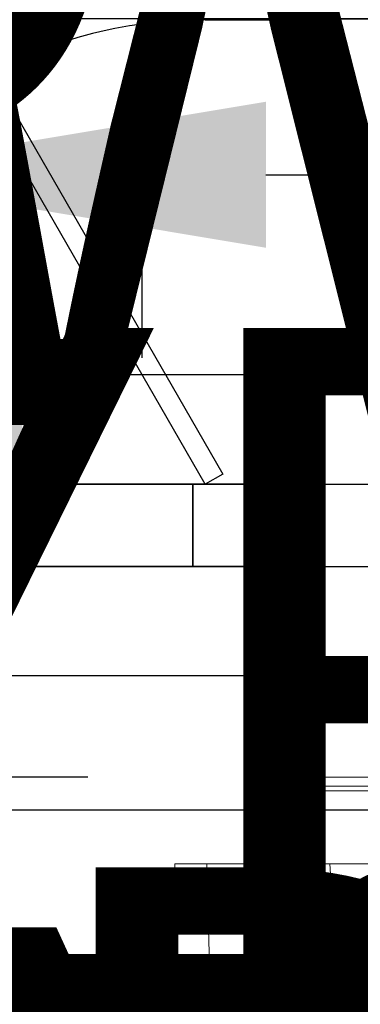
# Model space of a CAD drawing. Units: inches. Extents: x -307 to 2141, y -58 to 895.
# Tile 17 of 28: x 666 to 704, y 481 to 589. Entities that reach past the tile are written whole.
import ezdxf

# ---------------------------------------------------------------- set-up
doc = ezdxf.new("R2010")
doc.units = ezdxf.units.IN
doc.header["$MEASUREMENT"] = 0
for name, color, linetype, lineweight in [('A-ANNO-DIMS', 2, 'Continuous', 18), ('A-DOOR', 3, 'Continuous', 25), ('A-FURN', 8, 'Continuous', 18), ('A-WALL', 7, 'Continuous', 35)]:
    doc.layers.add(name, color=color, linetype=linetype, lineweight=lineweight)
doc.styles.get("Standard").update_dxf_attribs({"font": 'arial.ttf'})
doc.dimstyles.get("Standard").update_dxf_attribs({"dimtxt": 72, "dimasz": 48, "dimexe": 0.18, "dimexo": 0.0625, "dimgap": 0.09, "dimtad": 0, "dimtih": 1, "dimtoh": 1, "dimdec": 0, "dimrnd": 48, "dimzin": 0, "dimdsep": 46, "dimlunit": 3, "dimtxsty": 'Standard', "dimcen": 0.09, "dimadec": 0, "dimazin": 0, "dimtfac": 1, "dimtdec": 0, "dimtofl": 0, "dimtmove": 0, "dimatfit": 3, "dimfxl": 1, "dimtolj": 1, "dimtzin": 0, "dimarcsym": 0})

# ---------------------------------------------------------------- blocks, each defined once
blk = doc.blocks.new('*U3')
for p, q in [((-40, 0), (-40, 6)), ((0, 0), (0, 6))]:
    blk.add_line(p, q)
blk.add_lwpolyline([(0, 0), (-34.641, -20), (-35.516, -18.484), (-0.875, 1.516)], close=True)
blk.add_arc((0, 0), 40, 180, 210)
blk = doc.blocks.new('Dining Set - 36 x 72 in.')
for p, q in [((-22, 27.5), (-22.1562, 26.50042)), ((-22, 27.5), (-6, 27.5)), ((-5.8437, 26.49966), (-6, 27.5)), ((6, 27.5), (5.8438, 26.50042)), ((6, 27.5), (22, 27.5)), ((22.1563, 26.49966), (22, 27.5)), ((-22.2343, 26.00059), (-23.4847, 17.99762)), ((-22.2304, 26), (-5.7608, 26)), ((-5.8416, 26.5), (-22.1534, 26.5)), ((-4.5152, 17.99762), (-5.7655, 25.99926)), ((5.7657, 26.00059), (4.5153, 17.99762)), ((5.7696, 26), (22.2392, 26)), ((22.1584, 26.5), (5.8466, 26.5)), ((23.4848, 17.99762), (22.2345, 25.99926)), ((36, 18), (-36, 18)), ((-36, 18), (-36, -18)), ((36, -18), (36, 18)), ((-44.0006, 8.23428), (-35.9976, 9.48474)), ((44.0006, 8.23428), (35.9976, 9.48474)), ((-45.5, 8), (-44.5004, 8.15617)), ((-45.5, 8), (-45.5, -8)), ((-44.5, -8.15843), (-44.5, 8.15338)), ((-44, 8.23041), (-44, -8.23915)), ((44, 8.23041), (44, -8.23915)), ((44.5, -8.15843), (44.5, 8.15338)), ((45.5, 8), (44.5005, 8.15617)), ((45.5, 8), (45.5, -8)), ((-44.4997, -8.15631), (-45.5, -8)), ((-35.9976, -9.48476), (-43.9993, -8.2345)), ((35.9976, -9.48476), (43.9993, -8.2345)), ((44.4997, -8.15631), (45.5, -8)), ((-36, -18), (36, -18)), ((-22.2343, -26.0006), (-23.4847, -17.99762)), ((-4.5152, -17.99762), (-5.7655, -25.99928)), ((5.7657, -26.0006), (4.5153, -17.99762)), ((23.4848, -17.99762), (22.2345, -25.99928)), ((-22.2304, -26), (-5.7608, -26)), ((-22, -27.5), (-22.1562, -26.50044)), ((-5.8416, -26.5), (-22.1534, -26.5)), ((-5.8437, -26.49967), (-6, -27.5)), ((5.7696, -26), (22.2392, -26)), ((6, -27.5), (5.8438, -26.50044)), ((22.1584, -26.5), (5.8466, -26.5)), ((22.1563, -26.49967), (22, -27.5)), ((-22, -27.5), (-6, -27.5)), ((6, -27.5), (22, -27.5))]:
    blk.add_line(p, q)
for points in [[(-36, 15), (-31.1772, 14.97754), (-26.8079, 14.91406), (-22.8538, 14.81543), (-19.276, 14.6875), (-16.0362, 14.53613), (-13.0957, 14.36718), (-10.4159, 14.18652), (-7.9583, 14), (-5.6904, 13.81315), (-3.6035, 13.63021), (-1.6954, 13.45508), (0.0365, 13.29166), (1.5945, 13.14388), (2.9811, 13.01562), (4.1988, 12.9108), (5.25, 12.83333), (6.1393, 12.78613), (6.8802, 12.76823), (7.4883, 12.77767), (7.9792, 12.8125), (8.3685, 12.87077), (8.6719, 12.95052), (8.9049, 13.0498), (9.0833, 13.16666), (9.2205, 13.29899), (9.3216, 13.44401), (9.3895, 13.59879), (9.4271, 13.76041), (9.4373, 13.92594), (9.4232, 14.09245), (9.3875, 14.257), (9.3333, 14.41666), (9.2638, 14.56917), (9.1836, 14.71484), (9.0975, 14.85465), (9.0104, 14.98958), (8.9272, 15.1206), (8.8529, 15.2487), (8.7922, 15.37483), (8.75, 15.5), (8.7305, 15.62467), (8.7344, 15.74739), (8.7617, 15.86621), (8.8125, 15.97916), (8.8867, 16.08431), (8.9844, 16.17968), (9.1055, 16.26334), (9.25, 16.33333), (9.4189, 16.38802), (9.6172, 16.42708), (9.8506, 16.45052), (10.125, 16.45833), (10.4463, 16.45052), (10.8203, 16.42708), (11.2529, 16.38802), (11.75, 16.33333), (12.3184, 16.26318), (12.9694, 16.17838), (13.7151, 16.07991), (14.5677, 15.96875), (15.5395, 15.84586), (16.6426, 15.71224), (17.8893, 15.56884), (19.2917, 15.41666), (20.859, 15.25667), (22.5879, 15.08984), (24.4721, 14.91715), (26.5052, 14.73958), (28.6809, 14.5581), (30.9929, 14.3737), (33.4347, 14.18733), (36, 14)], [(-36, 10), (-28.9766, 10.14274), (-23.1725, 10.20442), (-18.4241, 10.19775), (-14.5677, 10.13541), (-11.4399, 10.03011), (-8.877, 9.89453), (-6.7154, 9.74137), (-4.7917, 9.58333), (-2.9698, 9.43082), (-1.2246, 9.28515), (0.4415, 9.14534), (2.026, 9.01041), (3.5266, 8.87939), (4.9408, 8.7513), (6.266, 8.62516), (7.5, 8.5), (8.6411, 8.37549), (9.6914, 8.2539), (10.6538, 8.13818), (11.5312, 8.03125), (12.3267, 7.93603), (13.043, 7.85547), (13.6831, 7.79248), (14.25, 7.75), (14.7471, 7.7303), (15.1797, 7.73307), (15.5537, 7.75732), (15.875, 7.80208), (16.1494, 7.86637), (16.3828, 7.94922), (16.5811, 8.04964), (16.75, 8.16666), (16.8944, 8.29915), (17.0143, 8.44531), (17.1089, 8.60319), (17.1771, 8.77083), (17.218, 8.94629), (17.2305, 9.1276), (17.2137, 9.31282), (17.1667, 9.5), (17.0895, 9.6875), (16.987, 9.875), (16.8649, 10.0625), (16.7292, 10.25), (16.5856, 10.4375), (16.4401, 10.625), (16.2985, 10.8125), (16.1667, 11), (16.05, 11.18733), (15.9518, 11.3737), (15.8752, 11.5581), (15.8229, 11.73958), (15.798, 11.91715), (15.8034, 12.08984), (15.842, 12.25667), (15.9167, 12.41666), (16.0295, 12.56836), (16.1784, 12.70833), (16.3605, 12.83268), (16.5729, 12.9375), (16.8127, 13.01888), (17.0768, 13.07291), (17.3625, 13.0957), (17.6667, 13.08333), (17.9894, 13.03312), (18.3418, 12.94726), (18.7382, 12.82918), (19.1927, 12.68229), (19.7195, 12.51001), (20.3327, 12.31575), (21.0465, 12.10294), (21.875, 11.875), (22.8357, 11.63354), (23.959, 11.37304), (25.2786, 11.08618), (26.8282, 10.76562), (28.6414, 10.40405), (30.752, 9.99414), (33.1936, 9.52856), (36, 9)], [(-36, 5.5), (-30.7157, 5.3348), (-26.069, 5.20963), (-21.9946, 5.11767), (-18.4271, 5.05208), (-15.3009, 5.00602), (-12.5508, 4.97265), (-10.1112, 4.94515), (-7.9167, 4.91666), (-5.909, 4.88167), (-4.0586, 4.83984), (-2.3429, 4.79215), (-0.7396, 4.73958), (0.7739, 4.6831), (2.22, 4.6237), (3.6213, 4.56233), (5, 4.5), (6.373, 4.43782), (7.7344, 4.3776), (9.0723, 4.32129), (10.375, 4.27083), (11.6309, 4.22819), (12.8281, 4.19531), (13.9551, 4.17415), (15, 4.16666), (15.954, 4.17448), (16.819, 4.19791), (17.6001, 4.23698), (18.3021, 4.29166), (18.9299, 4.36198), (19.4883, 4.44791), (19.9823, 4.54948), (20.4167, 4.66666), (20.7969, 4.79899), (21.1302, 4.94401), (21.4245, 5.09879), (21.6875, 5.26041), (21.9271, 5.42594), (22.1511, 5.59245), (22.3672, 5.757), (22.5834, 5.91666), (22.8065, 6.06868), (23.0404, 6.21093), (23.2879, 6.34147), (23.5521, 6.45833), (23.8358, 6.55957), (24.142, 6.64323), (24.4735, 6.70735), (24.8334, 6.75), (25.2235, 6.76969), (25.642, 6.76692), (26.0858, 6.74267), (26.5521, 6.69791), (27.0379, 6.63362), (27.5404, 6.55078), (28.0565, 6.45036), (28.5834, 6.33333), (29.1242, 6.19987), (29.7071, 6.04687), (30.3661, 5.87044), (31.1354, 5.66666), (32.0493, 5.43164), (33.142, 5.16146), (34.4475, 4.85221), (36, 4.5)], [(-36, -1), (-30.7915, -0.6591), (-26.0195, -0.38216), (-21.6519, -0.16284), (-17.6563, 0.00521), (-14.0005, 0.12833), (-10.6523, 0.21289), (-7.5796, 0.26522), (-4.75, 0.29166), (-2.134, 0.29793), (0.2878, 0.28711), (2.5317, 0.26163), (4.6146, 0.22396), (6.5529, 0.17651), (8.3633, 0.12174), (10.0623, 0.06209), (11.6667, 0), (13.1899, -0.06201), (14.6341, -0.1211), (15.9982, -0.17432), (17.2813, -0.21875), (18.4823, -0.25147), (19.6003, -0.26953), (20.6343, -0.27002), (21.5834, -0.25), (22.4481, -0.20768), (23.2357, -0.14584), (23.9549, -0.06836), (24.6146, 0.02083), (25.2235, 0.11784), (25.7904, 0.21875), (26.3241, 0.31966), (26.8334, 0.41666), (27.3265, 0.50618), (27.8099, 0.58593), (28.2894, 0.65397), (28.7709, 0.70833), (29.2601, 0.74707), (29.763, 0.76823), (30.2855, 0.76985), (30.8334, 0.75), (31.4088, 0.70784), (31.9994, 0.64713), (32.589, 0.57275), (33.1615, 0.48958), (33.7008, 0.4025), (34.1908, 0.3164), (34.6153, 0.23616), (34.9584, 0.16666), (35.2099, 0.11165), (35.3848, 0.07031), (35.504, 0.04069), (35.5886, 0.02083), (35.6594, 0.00879), (35.7377, 0.0026), (35.8442, 0.00032), (36, 0)], [(-36, -6.5), (-27.1843, -6.31267), (-20.084, -6.1263), (-14.469, -5.9419), (-10.1094, -5.76042), (-6.7752, -5.58285), (-4.2363, -5.41016), (-2.2629, -5.24333), (-0.625, -5.08334), (0.8708, -4.93099), (2.2715, -4.78646), (3.5872, -4.64974), (4.8281, -4.52084), (6.0046, -4.39974), (7.127, -4.28646), (8.2053, -4.18099), (9.25, -4.08334), (10.2705, -3.99382), (11.2734, -3.91407), (12.2647, -3.84603), (13.25, -3.79167), (14.2354, -3.75293), (15.2266, -3.73177), (16.2295, -3.73015), (17.25, -3.75), (18.2912, -3.79248), (19.3451, -3.85547), (20.4009, -3.93604), (21.4479, -4.03125), (22.4754, -4.13819), (23.4727, -4.25391), (24.4289, -4.37549), (25.3334, -4.5), (26.1785, -4.62492), (26.9694, -4.74935), (27.7145, -4.87281), (28.4219, -4.99479), (29.1, -5.11483), (29.7572, -5.23242), (30.4016, -5.34709), (31.0417, -5.45834), (31.6837, -5.56437), (32.3262, -5.65821), (32.9658, -5.73153), (33.599, -5.77604), (34.2224, -5.78345), (34.8327, -5.74545), (35.4264, -5.65373), (36, -5.5)], [(-36, -10), (-26.4022, -9.81299), (-18.4675, -9.62891), (-11.9839, -9.45069), (-6.7396, -9.28125), (-2.5226, -9.12354), (0.8789, -8.98047), (3.6769, -8.85498), (6.0833, -8.75), (8.2767, -8.66765), (10.3021, -8.60677), (12.1712, -8.56543), (13.8958, -8.54167), (15.4876, -8.53353), (16.9583, -8.53907), (18.3197, -8.55632), (19.5834, -8.58334), (20.7616, -8.61841), (21.8685, -8.66081), (22.9188, -8.71004), (23.9271, -8.76563), (24.9081, -8.82707), (25.8763, -8.89388), (26.8465, -8.96558), (27.8334, -9.04167), (28.8474, -9.12118), (29.8828, -9.20117), (30.93, -9.27824), (31.9792, -9.34896), (33.0205, -9.40991), (34.0443, -9.45768), (35.0407, -9.48885), (36, -9.5)], [(-36, -14.5), (-30.0881, -14.33513), (-25.0332, -14.21224), (-20.7312, -14.12647), (-17.0781, -14.07292), (-13.97, -14.04671), (-11.3027, -14.04297), (-8.9724, -14.05681), (-6.875, -14.08334), (-4.9224, -14.11833), (-3.0905, -14.16016), (-1.3709, -14.20785), (0.2448, -14.26042), (1.7647, -14.3169), (3.1973, -14.3763), (4.5507, -14.43767), (5.8333, -14.5), (7.0554, -14.5621), (8.235, -14.62175), (9.3922, -14.67652), (10.5469, -14.72396), (11.7192, -14.76164), (12.929, -14.78711), (14.1965, -14.79794), (15.5417, -14.79167), (16.9933, -14.76424), (18.6152, -14.70508), (20.4804, -14.60197), (22.6615, -14.44271), (25.2312, -14.21509), (28.2624, -13.9069), (31.8277, -13.50594), (36, -13)]]:
    blk.add_lwpolyline(points)
blk = doc.blocks.new('*D26')
at = {"layer": 'A-ANNO-DIMS', "color": 0, "lineweight": -2, "transparency": 16777216}
for p, q in [((565.34, 584.2), (565.34, 572.08)), ((645.34, 584.2), (645.34, 572.08)), ((517.34, 572.26), (469.34, 572.26)), ((693.34, 572.26), (741.34, 572.26))]:
    blk.add_line(p, q, dxfattribs=at)
at = {"layer": 'A-ANNO-DIMS', "color": 0, "transparency": 16777216}
for points in [[(517.34, 580.26), (517.34, 564.26), (565.34, 572.26)], [(693.34, 580.26), (693.34, 564.26), (645.34, 572.26)]]:
    blk.add_solid(points, dxfattribs=at)
at = {"layer": 'Defpoints', "color": 0, "transparency": 16777216}
for p in [(565.34, 584.26), (645.34, 584.26), (565.34, 572.26)]:
    blk.add_point(p, dxfattribs=at)
at = {"layer": 'A-ANNO-DIMS', "color": 0, "transparency": 16777216, "insert": (178.23, 572.26), "char_height": 72, "attachment_point": 5}
blk.add_mtext('\\A1;BED 80 TYP.', dxfattribs=at)
blk = doc.blocks.new('*D29')
at = {"layer": 'A-ANNO-DIMS', "color": 0, "lineweight": -2, "transparency": 16777216}
for p, q in [((747.42, 450.87), (699.42, 450.87)), ((795.42, 433.61), (795.42, 451.05)), ((882.03, 433.61), (882.03, 451.05)), ((930.03, 450.87), (978.03, 450.87))]:
    blk.add_line(p, q, dxfattribs=at)
at = {"layer": 'A-ANNO-DIMS', "color": 0, "transparency": 16777216}
for points in [[(747.42, 458.87), (747.42, 442.87), (795.42, 450.87)], [(930.03, 458.87), (930.03, 442.87), (882.03, 450.87)]]:
    blk.add_solid(points, dxfattribs=at)
at = {"layer": 'Defpoints', "color": 0, "transparency": 16777216}
for p in [(795.42, 450.87), (795.42, 433.55), (882.03, 433.55)]:
    blk.add_point(p, dxfattribs=at)
at = {"layer": 'A-ANNO-DIMS', "color": 0, "transparency": 16777216, "insert": (647.71, 450.87), "char_height": 72, "attachment_point": 5}
blk.add_mtext('\\A1;87', dxfattribs=at)
blk = doc.blocks.new('*D30')
at = {"layer": 'A-ANNO-DIMS', "color": 0, "lineweight": -2, "transparency": 16777216}
for p, q in [((570.74, 532.83), (570.74, 580.83)), ((570.74, 580.83), (618.74, 580.83)), ((565.4, 484.83), (570.92, 484.83)), ((565.4, 448.83), (570.92, 448.83)), ((570.74, 400.83), (570.74, 352.83))]:
    blk.add_line(p, q, dxfattribs=at)
at = {"layer": 'A-ANNO-DIMS', "color": 0, "transparency": 16777216}
for points in [[(562.74, 532.83), (578.74, 532.83), (570.74, 484.83)], [(562.74, 400.83), (578.74, 400.83), (570.74, 448.83)]]:
    blk.add_solid(points, dxfattribs=at)
at = {"layer": 'Defpoints', "color": 0, "transparency": 16777216}
for p in [(565.34, 484.83), (570.74, 484.83), (565.34, 448.83)]:
    blk.add_point(p, dxfattribs=at)
at = {"layer": 'A-ANNO-DIMS', "color": 0, "transparency": 16777216, "insert": (1030.17, 580.83), "char_height": 72, "attachment_point": 5}
blk.add_mtext('\\A1;WINDOW 36 TYP.', dxfattribs=at)
blk = doc.blocks.new('*D31')
at = {"layer": 'A-ANNO-DIMS', "color": 0, "lineweight": -2, "transparency": 16777216}
for p, q in [((556.34, 448.77), (556.34, 443.25)), ((565.34, 448.77), (565.34, 443.25)), ((508.34, 443.43), (460.34, 443.43)), ((613.34, 443.43), (661.34, 443.43))]:
    blk.add_line(p, q, dxfattribs=at)
at = {"layer": 'A-ANNO-DIMS', "color": 0, "transparency": 16777216}
for points in [[(508.34, 451.43), (508.34, 435.43), (556.34, 443.43)], [(613.34, 451.43), (613.34, 435.43), (565.34, 443.43)]]:
    blk.add_solid(points, dxfattribs=at)
at = {"layer": 'Defpoints', "color": 0, "transparency": 16777216}
for p in [(556.34, 448.83), (565.34, 448.83), (565.34, 443.43)]:
    blk.add_point(p, dxfattribs=at)
at = {"layer": 'A-ANNO-DIMS', "color": 0, "transparency": 16777216, "insert": (808.69, 443.43), "char_height": 72, "attachment_point": 5}
blk.add_mtext('\\A1;9 TYP.', dxfattribs=at)
blk = doc.blocks.new('*D35')
at = {"layer": 'A-ANNO-DIMS', "color": 0, "lineweight": -2, "transparency": 16777216}
for p, q in [((859.34, 453.77), (811.34, 453.77)), ((907.34, 443.03), (907.34, 453.95)), ((916.34, 443.03), (916.34, 453.95)), ((964.34, 453.77), (1012.34, 453.77))]:
    blk.add_line(p, q, dxfattribs=at)
at = {"layer": 'A-ANNO-DIMS', "color": 0, "transparency": 16777216}
for points in [[(859.34, 461.77), (859.34, 445.77), (907.34, 453.77)], [(964.34, 461.77), (964.34, 445.77), (916.34, 453.77)]]:
    blk.add_solid(points, dxfattribs=at)
at = {"layer": 'Defpoints', "color": 0, "transparency": 16777216}
for p in [(907.34, 453.77), (907.34, 442.97), (916.34, 442.97)]:
    blk.add_point(p, dxfattribs=at)
at = {"layer": 'A-ANNO-DIMS', "color": 0, "transparency": 16777216, "insert": (663.98, 453.77), "char_height": 72, "attachment_point": 5}
blk.add_mtext('\\A1;9 TYP.', dxfattribs=at)
blk = doc.blocks.new('*D36')
at = {"layer": 'A-ANNO-DIMS', "color": 0, "lineweight": -2, "transparency": 16777216}
for p, q in [((871.71, 562.4), (871.76, 610.4)), ((876.55, 514.4), (871.47, 514.4)), ((876.51, 481.35), (871.44, 481.36)), ((871.56, 433.36), (871.51, 385.36)), ((871.51, 385.36), (823.51, 385.36))]:
    blk.add_line(p, q, dxfattribs=at)
at = {"layer": 'A-ANNO-DIMS', "color": 0, "transparency": 16777216}
for points in [[(863.71, 562.41), (879.71, 562.4), (871.65, 514.4)], [(863.56, 433.37), (879.56, 433.35), (871.62, 481.36)]]:
    blk.add_solid(points, dxfattribs=at)
at = {"layer": 'Defpoints', "color": 0, "transparency": 16777216}
for p in [(876.61, 514.4), (871.62, 481.36), (876.57, 481.35)]:
    blk.add_point(p, dxfattribs=at)
at = {"layer": 'A-ANNO-DIMS', "color": 0, "transparency": 16777216, "insert": (548.95, 385.36), "char_height": 72, "attachment_point": 5}
blk.add_mtext('\\A1;WC 33 TYP.', dxfattribs=at)
blk = doc.blocks.new('*D37')
at = {"layer": 'A-ANNO-DIMS', "color": 0, "lineweight": -2, "transparency": 16777216}
for p, q in [((828.62, 519.41), (780.62, 519.46)), ((876.61, 514.46), (876.62, 519.54)), ((897.61, 514.44), (897.62, 519.51)), ((945.62, 519.28), (993.62, 519.22))]:
    blk.add_line(p, q, dxfattribs=at)
at = {"layer": 'A-ANNO-DIMS', "color": 0, "transparency": 16777216}
for points in [[(828.63, 527.41), (828.61, 511.41), (876.62, 519.36)], [(945.63, 527.28), (945.61, 511.28), (897.62, 519.33)]]:
    blk.add_solid(points, dxfattribs=at)
at = {"layer": 'Defpoints', "color": 0, "transparency": 16777216}
for p in [(876.62, 519.36), (876.61, 514.4), (897.61, 514.38)]:
    blk.add_point(p, dxfattribs=at)
at = {"layer": 'A-ANNO-DIMS', "color": 0, "transparency": 16777216, "insert": (604.68, 519.46), "char_height": 72, "attachment_point": 5}
blk.add_mtext('\\A1;21 TYP.', dxfattribs=at)
blk = doc.blocks.new('*D45')
at = {"layer": 'A-ANNO-DIMS', "color": 0, "lineweight": -2, "transparency": 16777216}
for p, q in [((841.11, 637.47), (793.11, 637.47)), ((842.12, 589.48), (841.11, 637.47)), ((839.51, 541.42), (843.31, 541.5)), ((839.93, 521.29), (843.73, 521.37)), ((844.56, 473.37), (845.57, 425.38))]:
    blk.add_line(p, q, dxfattribs=at)
at = {"layer": 'A-ANNO-DIMS', "color": 0, "transparency": 16777216}
for points in [[(850.12, 589.65), (834.12, 589.32), (843.13, 541.49)], [(852.56, 473.54), (836.56, 473.21), (843.55, 521.36)]]:
    blk.add_solid(points, dxfattribs=at)
at = {"layer": 'Defpoints', "color": 0, "transparency": 16777216}
for p in [(839.45, 541.42), (843.13, 541.49), (839.87, 521.29)]:
    blk.add_point(p, dxfattribs=at)
at = {"layer": 'A-ANNO-DIMS', "color": 0, "transparency": 16777216, "insert": (740.96, 637.47), "char_height": 72, "attachment_point": 5}
blk.add_mtext('\\A1;20', dxfattribs=at)
blk = doc.blocks.new('*D52')
at = {"layer": 'A-ANNO-DIMS', "color": 0, "lineweight": -2, "transparency": 16777216}
for p, q in [((660.21, 554.25), (660.21, 602.25)), ((673.8, 506.25), (660.03, 506.25)), ((673.8, 415.25), (660.03, 415.25)), ((660.21, 367.25), (660.21, 319.25))]:
    blk.add_line(p, q, dxfattribs=at)
at = {"layer": 'A-ANNO-DIMS', "color": 0, "transparency": 16777216}
for points in [[(652.21, 554.25), (668.21, 554.25), (660.21, 506.25)], [(652.21, 367.25), (668.21, 367.25), (660.21, 415.25)]]:
    blk.add_solid(points, dxfattribs=at)
at = {"layer": 'Defpoints', "color": 0, "transparency": 16777216}
for p in [(673.86, 506.25), (660.21, 415.25), (673.86, 415.25)]:
    blk.add_point(p, dxfattribs=at)
at = {"layer": 'A-ANNO-DIMS', "color": 0, "transparency": 16777216, "insert": (660.21, 460.75), "char_height": 72, "attachment_point": 5}
blk.add_mtext('\\A1;DINING SET 91', dxfattribs=at)
blk = doc.blocks.new('*D54')
at = {"layer": 'A-ANNO-DIMS', "color": 0, "lineweight": -2, "transparency": 16777216}
for p, q in [((605.34, 412.35), (605.34, 460.35)), ((605.34, 460.35), (653.34, 460.35)), ((596.4, 364.35), (605.52, 364.35)), ((596.4, 304.35), (605.52, 304.35)), ((605.34, 256.35), (605.34, 208.35))]:
    blk.add_line(p, q, dxfattribs=at)
at = {"layer": 'A-ANNO-DIMS', "color": 0, "transparency": 16777216}
for points in [[(597.34, 412.35), (613.34, 412.35), (605.34, 364.35)], [(597.34, 256.35), (613.34, 256.35), (605.34, 304.35)]]:
    blk.add_solid(points, dxfattribs=at)
at = {"layer": 'Defpoints', "color": 0, "transparency": 16777216}
for p in [(596.34, 364.35), (605.34, 364.35), (596.34, 304.35)]:
    blk.add_point(p, dxfattribs=at)
at = {"layer": 'A-ANNO-DIMS', "color": 0, "transparency": 16777216, "insert": (854, 460.35), "char_height": 72, "attachment_point": 5}
blk.add_mtext('\\A1;DESK 60', dxfattribs=at)
blk = doc.blocks.new('*D56')
at = {"layer": 'A-ANNO-DIMS', "color": 0, "lineweight": -2, "transparency": 16777216}
for p, q in [((679.73, 723.21), (679.73, 771.21)), ((679.73, 771.21), (727.73, 771.21)), ((675.74, 675.21), (679.91, 675.21)), ((675.74, 648.21), (679.91, 648.21)), ((679.73, 600.21), (679.73, 552.21))]:
    blk.add_line(p, q, dxfattribs=at)
at = {"layer": 'A-ANNO-DIMS', "color": 0, "transparency": 16777216}
for points in [[(671.73, 723.21), (687.73, 723.21), (679.73, 675.21)], [(671.73, 600.21), (687.73, 600.21), (679.73, 648.21)]]:
    blk.add_solid(points, dxfattribs=at)
at = {"layer": 'Defpoints', "color": 0, "transparency": 16777216}
for p in [(675.68, 675.21), (679.73, 675.21), (675.68, 648.21)]:
    blk.add_point(p, dxfattribs=at)
at = {"layer": 'A-ANNO-DIMS', "color": 0, "transparency": 16777216, "insert": (1006.66, 771.21), "char_height": 72, "attachment_point": 5}
blk.add_mtext('\\A1;ROCKER 27', dxfattribs=at)
blk = doc.blocks.new('*D62')
at = {"layer": 'A-ANNO-DIMS', "color": 0, "lineweight": -2, "transparency": 16777216}
for p, q in [((556.34, 691.4), (556.34, 722.72)), ((604.34, 722.54), (656.85, 722.54)), ((868.34, 722.54), (815.82, 722.54)), ((916.34, 490.97), (916.34, 722.72))]:
    blk.add_line(p, q, dxfattribs=at)
at = {"layer": 'A-ANNO-DIMS', "color": 0, "transparency": 16777216}
for points in [[(604.34, 730.54), (604.34, 714.54), (556.34, 722.54)], [(868.34, 730.54), (868.34, 714.54), (916.34, 722.54)]]:
    blk.add_solid(points, dxfattribs=at)
at = {"layer": 'Defpoints', "color": 0, "transparency": 16777216}
for p in [(916.34, 722.54), (556.34, 691.34), (916.34, 490.9)]:
    blk.add_point(p, dxfattribs=at)
at = {"layer": 'A-ANNO-DIMS', "color": 0, "transparency": 16777216, "insert": (736.34, 722.54), "char_height": 72, "attachment_point": 5}
blk.add_mtext('\\A1;360', dxfattribs=at)
blk = doc.blocks.new('*D68')
at = {"layer": 'A-ANNO-DIMS', "color": 0, "lineweight": -2, "transparency": 16777216}
for p, q in [((525.13, 586.34), (525.13, 634.34)), ((525.13, 634.34), (573.13, 634.34)), ((565.27, 538.34), (524.95, 538.34)), ((556.27, 484.83), (524.95, 484.83)), ((525.13, 436.83), (525.13, 388.83))]:
    blk.add_line(p, q, dxfattribs=at)
at = {"layer": 'A-ANNO-DIMS', "color": 0, "transparency": 16777216}
for points in [[(517.13, 586.34), (533.13, 586.34), (525.13, 538.34)], [(517.13, 436.83), (533.13, 436.83), (525.13, 484.83)]]:
    blk.add_solid(points, dxfattribs=at)
at = {"layer": 'Defpoints', "color": 0, "transparency": 16777216}
for p in [(525.13, 538.34), (565.34, 538.34), (556.34, 484.83)]:
    blk.add_point(p, dxfattribs=at)
at = {"layer": 'A-ANNO-DIMS', "color": 0, "transparency": 16777216, "insert": (687.75, 634.34), "char_height": 72, "attachment_point": 5}
blk.add_mtext('\\A1;53.51', dxfattribs=at)
blk = doc.blocks.new('*D69')
at = {"layer": 'A-ANNO-DIMS', "color": 0, "lineweight": -2, "transparency": 16777216}
for p, q in [((525.13, 682.34), (525.13, 730.34)), ((525.13, 730.34), (573.13, 730.34)), ((565.27, 682.34), (524.95, 682.34)), ((525.13, 586.34), (525.13, 634.34)), ((565.27, 538.34), (524.95, 538.34))]:
    blk.add_line(p, q, dxfattribs=at)
at = {"layer": 'A-ANNO-DIMS', "color": 0, "transparency": 16777216}
for points in [[(517.13, 634.34), (533.13, 634.34), (525.13, 682.34)], [(517.13, 586.34), (533.13, 586.34), (525.13, 538.34)]]:
    blk.add_solid(points, dxfattribs=at)
at = {"layer": 'Defpoints', "color": 0, "transparency": 16777216}
for p in [(525.13, 682.34), (565.34, 682.34), (565.34, 538.34)]:
    blk.add_point(p, dxfattribs=at)
at = {"layer": 'A-ANNO-DIMS', "color": 0, "transparency": 16777216, "insert": (649.22, 730.34), "char_height": 72, "attachment_point": 5}
blk.add_mtext('\\A1;144', dxfattribs=at)
blk = doc.blocks.new('*D82')
at = {"layer": 'A-ANNO-DIMS', "color": 0, "lineweight": -2, "transparency": 16777216}
for p, q in [((525.13, 565.34), (525.13, 613.34)), ((525.13, 613.34), (573.13, 613.34)), ((802.27, 517.34), (524.95, 517.34)), ((802.27, 481.34), (524.95, 481.34)), ((525.13, 433.34), (525.13, 385.34))]:
    blk.add_line(p, q, dxfattribs=at)
at = {"layer": 'A-ANNO-DIMS', "color": 0, "transparency": 16777216}
for points in [[(517.13, 565.34), (533.13, 565.34), (525.13, 517.34)], [(517.13, 433.34), (533.13, 433.34), (525.13, 481.34)]]:
    blk.add_solid(points, dxfattribs=at)
at = {"layer": 'Defpoints', "color": 0, "transparency": 16777216}
for p in [(525.13, 517.34), (802.34, 517.34), (802.34, 481.34)]:
    blk.add_point(p, dxfattribs=at)
at = {"layer": 'A-ANNO-DIMS', "color": 0, "transparency": 16777216, "insert": (624.74, 613.34), "char_height": 72, "attachment_point": 5}
blk.add_mtext('\\A1;36', dxfattribs=at)
blk = doc.blocks.new('*D83')
at = {"layer": 'A-ANNO-DIMS', "color": 0, "lineweight": -2, "transparency": 16777216}
for p, q in [((947.54, 538.9), (947.54, 586.9)), ((916.4, 490.9), (947.72, 490.9)), ((907.4, 481.34), (947.72, 481.34)), ((947.54, 433.34), (947.54, 385.34)), ((947.54, 385.34), (899.54, 385.34))]:
    blk.add_line(p, q, dxfattribs=at)
at = {"layer": 'A-ANNO-DIMS', "color": 0, "transparency": 16777216}
for points in [[(939.54, 538.9), (955.54, 538.9), (947.54, 490.9)], [(939.54, 433.34), (955.54, 433.34), (947.54, 481.34)]]:
    blk.add_solid(points, dxfattribs=at)
at = {"layer": 'Defpoints', "color": 0, "transparency": 16777216}
for p in [(916.34, 490.9), (907.34, 481.34), (947.54, 481.34)]:
    blk.add_point(p, dxfattribs=at)
at = {"layer": 'A-ANNO-DIMS', "color": 0, "transparency": 16777216, "insert": (777.97, 385.34), "char_height": 72, "attachment_point": 5}
blk.add_mtext('\\A1;9.563', dxfattribs=at)
blk = doc.blocks.new('*D88')
at = {"layer": 'A-ANNO-DIMS', "color": 0, "lineweight": -2, "transparency": 16777216}
for p, q in [((517.33584, 722.544828), (469.33584, 722.544828)), ((565.33584, 295.403328), (565.33584, 722.724828)), ((754.33584, 271.403328), (754.33584, 722.724828)), ((802.33584, 722.544828), (850.33584, 722.544828))]:
    blk.add_line(p, q, dxfattribs=at)
at = {"layer": 'A-ANNO-DIMS', "color": 0, "transparency": 16777216}
for points in [[(517.33584, 730.544828), (517.33584, 714.544828), (565.33584, 722.544828)], [(802.33584, 730.544828), (802.33584, 714.544828), (754.33584, 722.544828)]]:
    blk.add_solid(points, dxfattribs=at)
at = {"layer": 'Defpoints', "color": 0, "transparency": 16777216}
for p in [(754.33584, 722.544828), (565.33584, 295.340828), (754.33584, 271.340828)]:
    blk.add_point(p, dxfattribs=at)
at = {"layer": 'A-ANNO-DIMS', "color": 0, "transparency": 16777216, "insert": (659.83584, 722.544828), "char_height": 72, "attachment_point": 5}
blk.add_mtext('\\A1;189', dxfattribs=at)
blk = doc.blocks.new('*D94')
at = {"layer": 'A-ANNO-DIMS', "color": 0, "lineweight": -2, "transparency": 16777216}
for p, q in [((517.34, 722.54), (469.34, 722.54)), ((565.34, 529.4), (565.34, 722.72)), ((629.84, 529.4), (629.84, 722.72)), ((677.84, 722.54), (725.84, 722.54))]:
    blk.add_line(p, q, dxfattribs=at)
at = {"layer": 'A-ANNO-DIMS', "color": 0, "transparency": 16777216}
for points in [[(517.34, 730.54), (517.34, 714.54), (565.34, 722.54)], [(677.84, 730.54), (677.84, 714.54), (629.84, 722.54)]]:
    blk.add_solid(points, dxfattribs=at)
at = {"layer": 'Defpoints', "color": 0, "transparency": 16777216}
for p in [(629.84, 722.54), (565.34, 529.34), (629.84, 529.34)]:
    blk.add_point(p, dxfattribs=at)
at = {"layer": 'A-ANNO-DIMS', "color": 0, "transparency": 16777216, "insert": (819.9, 722.54), "char_height": 72, "attachment_point": 5}
blk.add_mtext('\\A1;64.5', dxfattribs=at)
blk = doc.blocks.new('*D95')
at = {"layer": 'A-ANNO-DIMS', "color": 0, "lineweight": -2, "transparency": 16777216}
for p, q in [((947.54, 577.34), (947.54, 625.34)), ((947.54, 625.34), (995.54, 625.34)), ((629.9, 529.34), (947.72, 529.34)), ((629.9, 502.66), (947.72, 502.66)), ((947.54, 454.66), (947.54, 406.66))]:
    blk.add_line(p, q, dxfattribs=at)
at = {"layer": 'A-ANNO-DIMS', "color": 0, "transparency": 16777216}
for points in [[(939.54, 577.34), (955.54, 577.34), (947.54, 529.34)], [(939.54, 454.66), (955.54, 454.66), (947.54, 502.66)]]:
    blk.add_solid(points, dxfattribs=at)
at = {"layer": 'Defpoints', "color": 0, "transparency": 16777216}
for p in [(629.84, 529.34), (947.54, 529.34), (629.84, 502.66)]:
    blk.add_point(p, dxfattribs=at)
at = {"layer": 'A-ANNO-DIMS', "color": 0, "transparency": 16777216, "insert": (1117.8, 625.34), "char_height": 72, "attachment_point": 5}
blk.add_mtext('\\A1;26.68', dxfattribs=at)
blk = doc.blocks.new('*D97')
at = {"layer": 'A-ANNO-DIMS', "color": 0, "lineweight": -2, "transparency": 16777216}
for p, q in [((947.54, 637.34), (947.54, 685.34)), ((947.54, 685.34), (995.54, 685.34)), ((685.4, 589.34), (947.72, 589.34)), ((685.4, 538.34), (947.72, 538.34)), ((947.54, 490.34), (947.54, 442.34))]:
    blk.add_line(p, q, dxfattribs=at)
at = {"layer": 'A-ANNO-DIMS', "color": 0, "transparency": 16777216}
for points in [[(939.54, 637.34), (955.54, 637.34), (947.54, 589.34)], [(939.54, 490.34), (955.54, 490.34), (947.54, 538.34)]]:
    blk.add_solid(points, dxfattribs=at)
at = {"layer": 'Defpoints', "color": 0, "transparency": 16777216}
for p in [(685.34, 589.34), (947.54, 589.34), (685.34, 538.34)]:
    blk.add_point(p, dxfattribs=at)
at = {"layer": 'A-ANNO-DIMS', "color": 0, "transparency": 16777216, "insert": (1040.25, 685.34), "char_height": 72, "attachment_point": 5}
blk.add_mtext('\\A1;51', dxfattribs=at)
blk = doc.blocks.new('*D98')
at = {"layer": 'A-ANNO-DIMS', "color": 0, "lineweight": -2, "transparency": 16777216}
for p, q in [((525.13, 637.34), (525.13, 685.34)), ((525.13, 685.34), (573.13, 685.34)), ((787.27, 589.34), (524.95, 589.34)), ((787.27, 550.34), (524.95, 550.34)), ((525.13, 502.34), (525.13, 454.34))]:
    blk.add_line(p, q, dxfattribs=at)
at = {"layer": 'A-ANNO-DIMS', "color": 0, "transparency": 16777216}
for points in [[(517.13, 637.34), (533.13, 637.34), (525.13, 589.34)], [(517.13, 502.34), (533.13, 502.34), (525.13, 550.34)]]:
    blk.add_solid(points, dxfattribs=at)
at = {"layer": 'Defpoints', "color": 0, "transparency": 16777216}
for p in [(525.13, 589.34), (787.34, 589.34), (787.34, 550.34)]:
    blk.add_point(p, dxfattribs=at)
at = {"layer": 'A-ANNO-DIMS', "color": 0, "transparency": 16777216, "insert": (624.84, 685.34), "char_height": 72, "attachment_point": 5}
blk.add_mtext('\\A1;39', dxfattribs=at)
blk = doc.blocks.new('*D107')
at = {"layer": 'A-ANNO-DIMS', "color": 0, "lineweight": -2, "transparency": 16777216}
for p, q in [((517.34, 722.54), (469.34, 722.54)), ((565.34, 409.4), (565.34, 722.72)), ((589.34, 409.4), (589.34, 722.72)), ((637.34, 722.54), (685.34, 722.54))]:
    blk.add_line(p, q, dxfattribs=at)
at = {"layer": 'A-ANNO-DIMS', "color": 0, "transparency": 16777216}
for points in [[(517.34, 730.54), (517.34, 714.54), (565.34, 722.54)], [(637.34, 730.54), (637.34, 714.54), (589.34, 722.54)]]:
    blk.add_solid(points, dxfattribs=at)
at = {"layer": 'Defpoints', "color": 0, "transparency": 16777216}
for p in [(589.34, 722.54), (565.34, 409.34), (589.34, 409.34)]:
    blk.add_point(p, dxfattribs=at)
at = {"layer": 'A-ANNO-DIMS', "color": 0, "transparency": 16777216, "insert": (835.49, 722.54), "char_height": 72, "attachment_point": 5}
blk.add_mtext('\\A1;24.003', dxfattribs=at)
blk = doc.blocks.new('*D108')
at = {"layer": 'A-ANNO-DIMS', "color": 0, "lineweight": -2, "transparency": 16777216}
for p, q in [((947.54, 550.66), (947.54, 598.66)), ((589.4, 502.66), (947.72, 502.66)), ((589.4, 409.34), (947.72, 409.34)), ((947.54, 361.34), (947.54, 313.34))]:
    blk.add_line(p, q, dxfattribs=at)
at = {"layer": 'A-ANNO-DIMS', "color": 0, "transparency": 16777216}
for points in [[(939.54, 550.66), (955.54, 550.66), (947.54, 502.66)], [(939.54, 361.34), (955.54, 361.34), (947.54, 409.34)]]:
    blk.add_solid(points, dxfattribs=at)
at = {"layer": 'Defpoints', "color": 0, "transparency": 16777216}
for p in [(589.34, 502.66), (947.54, 502.66), (589.34, 409.34)]:
    blk.add_point(p, dxfattribs=at)
at = {"layer": 'A-ANNO-DIMS', "color": 0, "transparency": 16777216, "insert": (947.54, 456), "char_height": 72, "attachment_point": 5}
blk.add_mtext('\\A1;93.32', dxfattribs=at)

msp = doc.modelspace()

# ---------------------------------------------------------------- linework, layer by layer
at = {"layer": 'A-WALL'}
for p, q in [((694.3358, 538.3408), (565.3358, 538.3408)), ((685.3358, 538.3408), (685.3358, 529.3408)), ((694.3358, 538.3408), (694.3358, 529.3408)), ((694.3358, 529.3408), (565.3358, 529.3408))]:
    msp.add_line(p, q, dxfattribs=at)

# ---------------------------------------------------------------- block references
at = {"layer": 'A-DOOR', "xscale": 1.272826874134829, "yscale": 1.272826874134829, "zscale": 1.272826874134829, "rotation": 270}
msp.add_blockref('*U3', (686.6989, 538.3408), dxfattribs=at)
at = {"layer": 'A-FURN', "rotation": 270}
msp.add_blockref('Dining Set - 36 x 72 in.', (701.3583, 460.7485), dxfattribs=at)

# ---------------------------------------------------------------- dimensions: what is measured, and where the dimension line sits
at = {"layer": 'A-ANNO-DIMS'}
for base, p1, p2, angle, text, picture, middle in [((679.7317, 675.211), (675.6817, 648.211), (675.6817, 675.211), 90, 'ROCKER <>', '*D56', (1006.6621, 771.211)), ((570.7358, 484.8333), (565.3358, 448.8333), (565.3358, 484.8333), 90, 'WINDOW <> TYP.', '*D30', (1030.1737, 580.8333)), ((565.3358, 572.2648), (645.3359, 584.2648), (565.3358, 584.2648), 180, 'BED <> TYP.', '*D26', (178.2254, 572.2648)), ((660.2083, 415.2485), (673.8583, 506.2485), (673.8583, 415.2485), 270, 'DINING SET <>', '*D52', (660.2083, 460.7485)), ((876.6162, 519.3557), (897.6106, 514.3753), (876.6106, 514.3988), 179.935892, '<> TYP.', '*D37', (604.6763, 519.4631)), ((871.6167, 481.3581), (876.6106, 514.3988), (876.5736, 481.3526), 269.935892, 'WC <> TYP.', '*D36', (548.95, 385.3582)), ((605.3358, 364.3488), (596.3358, 304.3488), (596.3358, 364.3488), 90, 'DESK <>', '*D54', (854.0043, 460.3488)), ((907.3358, 453.7692), (916.3358, 442.9669), (907.3358, 442.9669), 180, '<> TYP.', '*D35', (663.9798, 453.7692))]:
    dim = msp.add_linear_dim(base=base, p1=p1, p2=p2, angle=angle, text=text, dimstyle='Standard', override={"dimdec": 0, "dimlfac": 1, "dimrnd": 0, "dimzin": 0, "dimdsep": 46, "dimlunit": 2}, dxfattribs=at)
    dim.commit()
    dim.dimension.update_dxf_attribs({"geometry": picture, "text_midpoint": middle})
for base, p1, p2, angle, override, picture, middle in [((525.1318, 682.3408), (565.3358, 538.3408), (565.3358, 682.3408), 90, {"dimdec": 0, "dimlfac": 1, "dimrnd": 0, "dimzin": 0, "dimdsep": 46, "dimlunit": 2}, '*D69', (649.2246, 730.3408)), ((525.1318, 589.3408), (787.3358, 550.3408), (787.3358, 589.3408), 90, {"dimdec": 0, "dimlfac": 1, "dimrnd": 0, "dimzin": 0, "dimdsep": 46, "dimlunit": 2}, '*D98', (624.8398, 685.3408)), ((947.5398, 589.3408), (685.3358, 538.3408), (685.3358, 589.3408), 90, {"dimdec": 0, "dimlfac": 1, "dimrnd": 0, "dimzin": 0, "dimdsep": 46, "dimlunit": 2}, '*D97', (1040.2492, 685.3408)), ((843.1292, 541.4949), (839.8707, 521.2853), (839.4474, 541.4175), 91.204628, {"dimdec": 0, "dimlfac": 1, "dimrnd": 0, "dimzin": 0, "dimdsep": 46, "dimlunit": 2}, '*D45', (740.961, 637.4737)), ((525.1318, 538.3408), (556.3358, 484.8333), (565.3358, 538.3408), 90, {"dimdec": 2, "dimlfac": 1, "dimrnd": 0, "dimzin": 0, "dimdsep": 46, "dimlunit": 2}, '*D68', (687.7539, 634.3408)), ((947.5398, 529.3408), (629.8358, 502.6632), (629.8358, 529.3408), 90, {"dimdec": 2, "dimlfac": 1, "dimrnd": 0, "dimzin": 0, "dimdsep": 46, "dimlunit": 2}, '*D95', (1117.799, 625.3408)), ((525.1318, 517.3408), (802.3358, 481.3408), (802.3358, 517.3408), 90, {"dimdec": 0, "dimlfac": 1, "dimrnd": 0, "dimzin": 0, "dimdsep": 46, "dimlunit": 2}, '*D82', (624.7416, 613.3408)), ((947.5398, 502.6632), (589.339, 409.3408), (589.339, 502.6632), 90, {"dimdec": 2, "dimlfac": 1, "dimrnd": 0, "dimzin": 0, "dimdsep": 46, "dimlunit": 2}, '*D108', (947.5398, 456.002)), ((947.5398, 481.3408), (916.3358, 490.9034), (907.3358, 481.3408), 90, {"dimdec": 3, "dimlfac": 1, "dimrnd": 0, "dimzin": 0, "dimdsep": 46, "dimlunit": 2}, '*D83', (777.9683, 385.3408)), ((795.4208, 450.8711), (882.0282, 433.5496), (795.4208, 433.5496), 180, {"dimdec": 0, "dimlfac": 1, "dimrnd": 0, "dimzin": 0, "dimdsep": 46, "dimlunit": 2}, '*D29', (647.7128, 450.8711))]:
    dim = msp.add_linear_dim(base=base, p1=p1, p2=p2, angle=angle, dimstyle='Standard', override=override, dxfattribs=at)
    dim.commit()
    dim.dimension.update_dxf_attribs({"geometry": picture, "text_midpoint": middle})
for base, p1, p2, override, picture, middle in [((754.3358, 722.5448), (565.3358, 295.3408), (754.3358, 271.3408), {"dimdec": 0, "dimlfac": 1, "dimrnd": 0, "dimzin": 0, "dimdsep": 46, "dimlunit": 2}, '*D88', (659.8358, 722.5448)), ((629.8358, 722.5448), (565.3358, 529.3408), (629.8358, 529.3408), {"dimdec": 1, "dimlfac": 1, "dimrnd": 0, "dimzin": 0, "dimdsep": 46, "dimlunit": 2}, '*D94', (819.904, 722.5448)), ((589.339, 722.5448), (565.3358, 409.3408), (589.339, 409.3408), {"dimdec": 3, "dimlfac": 1, "dimrnd": 0, "dimzin": 0, "dimdsep": 46, "dimlunit": 2}, '*D107', (835.4945, 722.5448)), ((916.3358, 722.5448), (556.3358, 691.3408), (916.3358, 490.9034), {"dimdec": 0, "dimlfac": 1, "dimrnd": 0, "dimzin": 0, "dimdsep": 46, "dimlunit": 2}, '*D62', (736.3358, 722.5448))]:
    dim = msp.add_linear_dim(base=base, p1=p1, p2=p2, dimstyle='Standard', override=override, dxfattribs=at)
    dim.commit()
    dim.dimension.update_dxf_attribs({"geometry": picture, "text_midpoint": middle})
dim = msp.add_linear_dim(base=(565.3358, 443.4333), p1=(556.3358, 448.8333), p2=(565.3358, 448.8333), text='<> TYP.', dimstyle='Standard', override={"dimdec": 0, "dimlfac": 1, "dimrnd": 0, "dimzin": 0, "dimdsep": 46, "dimlunit": 2}, dxfattribs=at)
dim.commit()
dim.dimension.update_dxf_attribs({"geometry": '*D31', "text_midpoint": (808.6919, 443.4333)})

doc.saveas('drawing.dxf')
